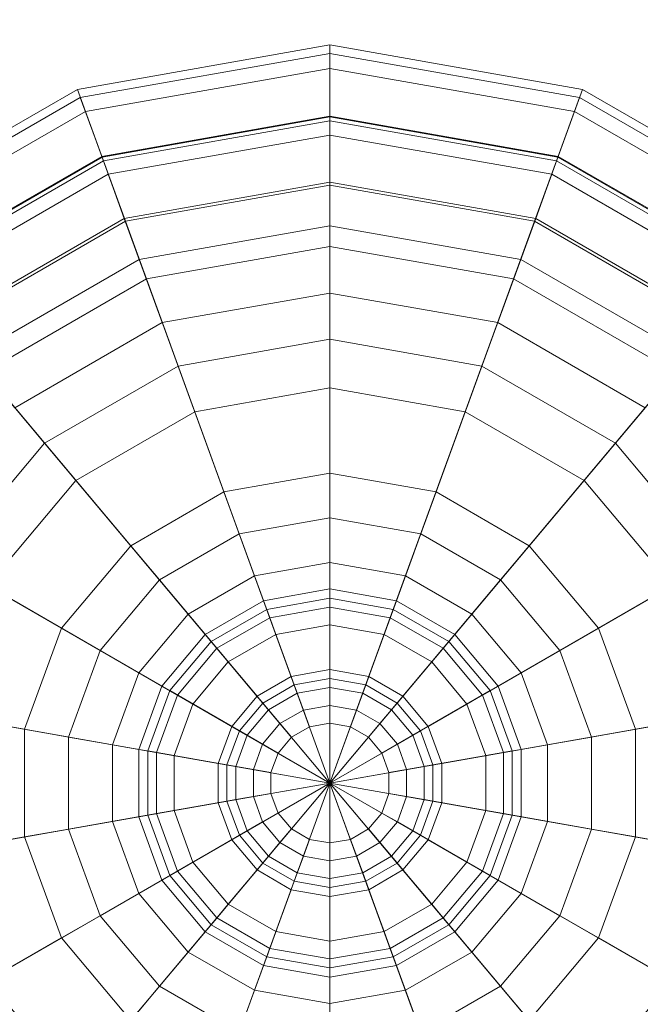
# Model space of a CAD drawing. Units: inches. Extents: x 375 to 1122, y 27 to 1069.
# Tile 92 of 155: x 729.113 to 730.25, y 860.072 to 861.878. Entities that reach past the tile are written whole.
import ezdxf

# ---------------------------------------------------------------- set-up
doc = ezdxf.new("R2010")
doc.units = ezdxf.units.IN
doc.layers.add('A-ANNO-DIMS', color=2, linetype='Continuous', lineweight=18)
doc.layers.add('Furniture', color=30, linetype='Continuous', lineweight=18)
doc.styles.get("Standard").update_dxf_attribs({"font": 'arial.ttf'})
doc.dimstyles.new('ISO-25', dxfattribs={"dimtxt": 12, "dimasz": 2.5, "dimexe": 1.5, "dimexo": 1.5, "dimtad": 1, "dimdec": 1, "dimlunit": 3, "dimtxsty": 'Standard', "dimblk": 'ARCHTICK', "dimcen": 2.5, "dimadec": 0, "dimazin": 0, "dimtfac": 1, "dimtdec": 1, "dimtmove": 0, "dimatfit": 3, "dimfxl": 1.5, "dimfxlon": 1, "dimarcsym": 0})

# ---------------------------------------------------------------- blocks, each defined once
blk = doc.blocks.new('A$C403C54AD')
for points in [[(1.940462, 1.15174, -0.060915), (1.946342, 1.118392, -0.057836), (1.946342, 1.118392, -0.057836), (1.929411, 1.147718, -0.060915)], [(1.952223, 1.15174, -0.060915), (1.946342, 1.118392, -0.057836), (1.946342, 1.118392, -0.057836), (1.940462, 1.15174, -0.060915)], [(1.963274, 1.147718, -0.060915), (1.946342, 1.118392, -0.057836), (1.946342, 1.118392, -0.057836), (1.952223, 1.15174, -0.060915)], [(1.943874, 1.13239, -0.054409), (1.941029, 1.148524, -0.057684), (1.931044, 1.144889, -0.057684), (1.939235, 1.130702, -0.054409)], [(1.948811, 1.13239, -0.054409), (1.951655, 1.148524, -0.057684), (1.941029, 1.148524, -0.057684), (1.943874, 1.13239, -0.054409)], [(1.95345, 1.130702, -0.054409), (1.961641, 1.144889, -0.057684), (1.951655, 1.148524, -0.057684), (1.948811, 1.13239, -0.054409)], [(1.929411, 1.147718, -0.060915), (1.946342, 1.118392, -0.057836), (1.946342, 1.118392, -0.057836), (1.920403, 1.140158, -0.060915)], [(1.972282, 1.140158, -0.060915), (1.946342, 1.118392, -0.057836), (1.946342, 1.118392, -0.057836), (1.963274, 1.147718, -0.060915)], [(1.939235, 1.130702, -0.054409), (1.931044, 1.144889, -0.057684), (1.922904, 1.138059, -0.057684), (1.935454, 1.127529, -0.054409)], [(1.957231, 1.127529, -0.054409), (1.969781, 1.138059, -0.057684), (1.961641, 1.144889, -0.057684), (1.95345, 1.130702, -0.054409)], [(1.932631, 1.142142, 0.042594), (1.936164, 1.136022, 0.032362), (1.930748, 1.131478, 0.032362), (1.925335, 1.13602, 0.042594)], [(1.920403, 1.140158, -0.060915), (1.946342, 1.118392, -0.057836), (1.946342, 1.118392, -0.057836), (1.914522, 1.129974, -0.060915)], [(1.922904, 1.138059, -0.057684), (1.920403, 1.140158, -0.060915), (1.914522, 1.129974, -0.060915), (1.917591, 1.128857, -0.057684)], [(1.978163, 1.129974, -0.060915), (1.946342, 1.118392, -0.057836), (1.946342, 1.118392, -0.057836), (1.972282, 1.140158, -0.060915)], [(1.922935, 1.138033, 0.102069), (1.920708, 1.139902, 0.088845), (1.914897, 1.129837, 0.088845), (1.917629, 1.128843, 0.102069)], [(1.920708, 1.139902, 0.088845), (1.921225, 1.139468, 0.060603), (1.915531, 1.129606, 0.060603), (1.914897, 1.129837, 0.088845)], [(1.937279, 1.134091, 0.03455), (1.934036, 1.139708, 0.043942), (1.927488, 1.134213, 0.043942), (1.932456, 1.130044, 0.03455)], [(1.960229, 1.130044, 0.03455), (1.965197, 1.134213, 0.043942), (1.958649, 1.139708, 0.043942), (1.955406, 1.134091, 0.03455)], [(1.921225, 1.139468, 0.060603), (1.925335, 1.13602, 0.042594), (1.920572, 1.127772, 0.042594), (1.915531, 1.129606, 0.060603)], [(1.942807, 1.13844, 0.032362), (1.944585, 1.128357, 0.024995), (1.941283, 1.127155, 0.024995), (1.936164, 1.136022, 0.032362)], [(1.949878, 1.13844, 0.032362), (1.9481, 1.128357, 0.024995), (1.944585, 1.128357, 0.024995), (1.942807, 1.13844, 0.032362)], [(1.956521, 1.136022, 0.032362), (1.951402, 1.127155, 0.024995), (1.9481, 1.128357, 0.024995), (1.949878, 1.13844, 0.032362)], [(1.935454, 1.127529, -0.054409), (1.922904, 1.138059, -0.057684), (1.917591, 1.128857, -0.057684), (1.932985, 1.123254, -0.054409)], [(1.926763, 1.134821, 0.111475), (1.922935, 1.138033, 0.102069), (1.917629, 1.128843, 0.102069), (1.922324, 1.127134, 0.111475)], [(1.923071, 1.137919, 0.088628), (1.925223, 1.136113, 0.101264), (1.920436, 1.127821, 0.101264), (1.917796, 1.128782, 0.088628)], [(1.923575, 1.137496, 0.061088), (1.923071, 1.137919, 0.088628), (1.917796, 1.128782, 0.088628), (1.918414, 1.128557, 0.061088)], [(1.927488, 1.134213, 0.043942), (1.923575, 1.137496, 0.061088), (1.918414, 1.128557, 0.061088), (1.923214, 1.12681, 0.043942)], [(1.925223, 1.136113, 0.101264), (1.929121, 1.132843, 0.111475), (1.925217, 1.126081, 0.111475), (1.920436, 1.127821, 0.101264)], [(1.936164, 1.136022, 0.032362), (1.941283, 1.127155, 0.024995), (1.938591, 1.124896, 0.024995), (1.930748, 1.131478, 0.032362)], [(1.944796, 1.127161, 0.027913), (1.943195, 1.136244, 0.03455), (1.937279, 1.134091, 0.03455), (1.94189, 1.126103, 0.027913)], [(1.947889, 1.127161, 0.027913), (1.94949, 1.136244, 0.03455), (1.943195, 1.136244, 0.03455), (1.944796, 1.127161, 0.027913)], [(1.950795, 1.126103, 0.027913), (1.955406, 1.134091, 0.03455), (1.94949, 1.136244, 0.03455), (1.947889, 1.127161, 0.027913)], [(1.961937, 1.131478, 0.032362), (1.954094, 1.124896, 0.024995), (1.951402, 1.127155, 0.024995), (1.956521, 1.136022, 0.032362)], [(1.925335, 1.13602, 0.042594), (1.930748, 1.131478, 0.032362), (1.927213, 1.125355, 0.032362), (1.920572, 1.127772, 0.042594)], [(1.929121, 1.132843, 0.111475), (1.926763, 1.134821, 0.111475), (1.922324, 1.127134, 0.111475), (1.925217, 1.126081, 0.111475)], [(1.932456, 1.130044, 0.03455), (1.927488, 1.134213, 0.043942), (1.923214, 1.12681, 0.043942), (1.929308, 1.124592, 0.03455)], [(1.94189, 1.126103, 0.027913), (1.937279, 1.134091, 0.03455), (1.932456, 1.130044, 0.03455), (1.939522, 1.124116, 0.027913)], [(1.953163, 1.124116, 0.027913), (1.960229, 1.130044, 0.03455), (1.955406, 1.134091, 0.03455), (1.950795, 1.126103, 0.027913)], [(1.94423, 1.130374, -0.051544), (1.943874, 1.13239, -0.054409), (1.939235, 1.130702, -0.054409), (1.940259, 1.128929, -0.051544)], [(1.948455, 1.130374, -0.051544), (1.948811, 1.13239, -0.054409), (1.943874, 1.13239, -0.054409), (1.94423, 1.130374, -0.051544)], [(1.952426, 1.128929, -0.051544), (1.95345, 1.130702, -0.054409), (1.948811, 1.13239, -0.054409), (1.948455, 1.130374, -0.051544)], [(1.930748, 1.131478, 0.032362), (1.938591, 1.124896, 0.024995), (1.936834, 1.121853, 0.024995), (1.927213, 1.125355, 0.032362)], [(1.965472, 1.125355, 0.032362), (1.955851, 1.121853, 0.024995), (1.954094, 1.124896, 0.024995), (1.961937, 1.131478, 0.032362)], [(1.940259, 1.128929, -0.051544), (1.939235, 1.130702, -0.054409), (1.935454, 1.127529, -0.054409), (1.937022, 1.126213, -0.051544)], [(1.955663, 1.126213, -0.051544), (1.957231, 1.127529, -0.054409), (1.95345, 1.130702, -0.054409), (1.952426, 1.128929, -0.051544)], [(1.944941, 1.12634, -0.049498), (1.94423, 1.130374, -0.051544), (1.940259, 1.128929, -0.051544), (1.942307, 1.125382, -0.049498)], [(1.947744, 1.12634, -0.049498), (1.948455, 1.130374, -0.051544), (1.94423, 1.130374, -0.051544), (1.944941, 1.12634, -0.049498)], [(1.950378, 1.125382, -0.049498), (1.952426, 1.128929, -0.051544), (1.948455, 1.130374, -0.051544), (1.947744, 1.12634, -0.049498)], [(1.914522, 1.129974, -0.060915), (1.946342, 1.118392, -0.057836), (1.946342, 1.118392, -0.057836), (1.91248, 1.118392, -0.060915)], [(1.917591, 1.128857, -0.057684), (1.914522, 1.129974, -0.060915), (1.91248, 1.118392, -0.060915), (1.915746, 1.118392, -0.057684)], [(1.917629, 1.128843, 0.102069), (1.914897, 1.129837, 0.088845), (1.912879, 1.118392, 0.088845), (1.915786, 1.118392, 0.102069)], [(1.914897, 1.129837, 0.088845), (1.915531, 1.129606, 0.060603), (1.913554, 1.118392, 0.060603), (1.912879, 1.118392, 0.088845)], [(1.939522, 1.124116, 0.027913), (1.932456, 1.130044, 0.03455), (1.929308, 1.124592, 0.03455), (1.937975, 1.121437, 0.027913)], [(1.980205, 1.118392, -0.060915), (1.946342, 1.118392, -0.057836), (1.946342, 1.118392, -0.057836), (1.978163, 1.129974, -0.060915)], [(1.95471, 1.121437, 0.027913), (1.963376, 1.124592, 0.03455), (1.960229, 1.130044, 0.03455), (1.953163, 1.124116, 0.027913)], [(1.915531, 1.129606, 0.060603), (1.920572, 1.127772, 0.042594), (1.918919, 1.118392, 0.042594), (1.913554, 1.118392, 0.060603)], [(1.932985, 1.123254, -0.054409), (1.917591, 1.128857, -0.057684), (1.915746, 1.118392, -0.057684), (1.932128, 1.118392, -0.054409)], [(1.922324, 1.127134, 0.111475), (1.917629, 1.128843, 0.102069), (1.915786, 1.118392, 0.102069), (1.920783, 1.118392, 0.111475)], [(1.942307, 1.125382, -0.049498), (1.940259, 1.128929, -0.051544), (1.937022, 1.126213, -0.051544), (1.94016, 1.12358, -0.049498)], [(1.952525, 1.12358, -0.049498), (1.955663, 1.126213, -0.051544), (1.952426, 1.128929, -0.051544), (1.950378, 1.125382, -0.049498)], [(1.917796, 1.128782, 0.088628), (1.920436, 1.127821, 0.101264), (1.918773, 1.118392, 0.101264), (1.915964, 1.118392, 0.088628)], [(1.918414, 1.128557, 0.061088), (1.917796, 1.128782, 0.088628), (1.915964, 1.118392, 0.088628), (1.916622, 1.118392, 0.061088)], [(1.923214, 1.12681, 0.043942), (1.918414, 1.128557, 0.061088), (1.916622, 1.118392, 0.061088), (1.921729, 1.118392, 0.043942)], [(1.944585, 1.128357, 0.024995), (1.945439, 1.123517, 0.024176), (1.94374, 1.122899, 0.024176), (1.941283, 1.127155, 0.024995)], [(1.9481, 1.128357, 0.024995), (1.947246, 1.123517, 0.024176), (1.945439, 1.123517, 0.024176), (1.944585, 1.128357, 0.024995)], [(1.951402, 1.127155, 0.024995), (1.948945, 1.122899, 0.024176), (1.947246, 1.123517, 0.024176), (1.9481, 1.128357, 0.024995)], [(1.920436, 1.127821, 0.101264), (1.925217, 1.126081, 0.111475), (1.923861, 1.118392, 0.111475), (1.918773, 1.118392, 0.101264)], [(1.920572, 1.127772, 0.042594), (1.927213, 1.125355, 0.032362), (1.925985, 1.118392, 0.032362), (1.918919, 1.118392, 0.042594)], [(1.937022, 1.126213, -0.051544), (1.935454, 1.127529, -0.054409), (1.932985, 1.123254, -0.054409), (1.93491, 1.122553, -0.051544)], [(1.957775, 1.122553, -0.051544), (1.9597, 1.123254, -0.054409), (1.957231, 1.127529, -0.054409), (1.955663, 1.126213, -0.051544)], [(1.925217, 1.126081, 0.111475), (1.922324, 1.127134, 0.111475), (1.920783, 1.118392, 0.111475), (1.923861, 1.118392, 0.111475)], [(1.941283, 1.127155, 0.024995), (1.94374, 1.122899, 0.024176), (1.942356, 1.121737, 0.024176), (1.938591, 1.124896, 0.024995)], [(1.946342, 1.118392, 0.02643), (1.944796, 1.127161, 0.027913), (1.94189, 1.126103, 0.027913), (1.946342, 1.118392, 0.02643)], [(1.946342, 1.118392, 0.02643), (1.947889, 1.127161, 0.027913), (1.944796, 1.127161, 0.027913), (1.946342, 1.118392, 0.02643)], [(1.946342, 1.118392, 0.02643), (1.950795, 1.126103, 0.027913), (1.947889, 1.127161, 0.027913), (1.946342, 1.118392, 0.02643)], [(1.954094, 1.124896, 0.024995), (1.950329, 1.121737, 0.024176), (1.948945, 1.122899, 0.024176), (1.951402, 1.127155, 0.024995)], [(1.929308, 1.124592, 0.03455), (1.923214, 1.12681, 0.043942), (1.921729, 1.118392, 0.043942), (1.928215, 1.118392, 0.03455)], [(1.94487, 1.126744, 0.021311), (1.945581, 1.122711, 0.019264), (1.94415, 1.12219, 0.019264), (1.942102, 1.125736, 0.021311)], [(1.945083, 1.125534, 0.023357), (1.94487, 1.126744, 0.021311), (1.942102, 1.125736, 0.021311), (1.942717, 1.124672, 0.023357)], [(1.947815, 1.126744, 0.021311), (1.947104, 1.122711, 0.019264), (1.945581, 1.122711, 0.019264), (1.94487, 1.126744, 0.021311)], [(1.947602, 1.125534, 0.023357), (1.947815, 1.126744, 0.021311), (1.94487, 1.126744, 0.021311), (1.945083, 1.125534, 0.023357)], [(1.950583, 1.125736, 0.021311), (1.948535, 1.12219, 0.019264), (1.947104, 1.122711, 0.019264), (1.947815, 1.126744, 0.021311)], [(1.949968, 1.124672, 0.023357), (1.950583, 1.125736, 0.021311), (1.947815, 1.126744, 0.021311), (1.947602, 1.125534, 0.023357)], [(1.94016, 1.12358, -0.049498), (1.937022, 1.126213, -0.051544), (1.93491, 1.122553, -0.051544), (1.938758, 1.121153, -0.049498)], [(1.946342, 1.118392, 0.02643), (1.94189, 1.126103, 0.027913), (1.939522, 1.124116, 0.027913), (1.946342, 1.118392, 0.02643)], [(1.94551, 1.123114, -0.044177), (1.944941, 1.12634, -0.049498), (1.942307, 1.125382, -0.049498), (1.943945, 1.122544, -0.044177)], [(1.947175, 1.123114, -0.044177), (1.947744, 1.12634, -0.049498), (1.944941, 1.12634, -0.049498), (1.94551, 1.123114, -0.044177)], [(1.946342, 1.118392, 0.02643), (1.953163, 1.124116, 0.027913), (1.950795, 1.126103, 0.027913), (1.946342, 1.118392, 0.02643)], [(1.94874, 1.122544, -0.044177), (1.950378, 1.125382, -0.049498), (1.947744, 1.12634, -0.049498), (1.947175, 1.123114, -0.044177)], [(1.953927, 1.121153, -0.049498), (1.957775, 1.122553, -0.051544), (1.955663, 1.126213, -0.051544), (1.952525, 1.12358, -0.049498)], [(1.942102, 1.125736, 0.021311), (1.94415, 1.12219, 0.019264), (1.942983, 1.121211, 0.019264), (1.939846, 1.123843, 0.021311)], [(1.942717, 1.124672, 0.023357), (1.942102, 1.125736, 0.021311), (1.939846, 1.123843, 0.021311), (1.940787, 1.123054, 0.023357)], [(1.952839, 1.123843, 0.021311), (1.949702, 1.121211, 0.019264), (1.948535, 1.12219, 0.019264), (1.950583, 1.125736, 0.021311)], [(1.951898, 1.123054, 0.023357), (1.952839, 1.123843, 0.021311), (1.950583, 1.125736, 0.021311), (1.949968, 1.124672, 0.023357)], [(1.927213, 1.125355, 0.032362), (1.936834, 1.121853, 0.024995), (1.936224, 1.118392, 0.024995), (1.925985, 1.118392, 0.032362)], [(1.943945, 1.122544, -0.044177), (1.942307, 1.125382, -0.049498), (1.94016, 1.12358, -0.049498), (1.94267, 1.121474, -0.044177)], [(1.945439, 1.123517, 0.024176), (1.945083, 1.125534, 0.023357), (1.942717, 1.124672, 0.023357), (1.94374, 1.122899, 0.024176)], [(1.947246, 1.123517, 0.024176), (1.947602, 1.125534, 0.023357), (1.945083, 1.125534, 0.023357), (1.945439, 1.123517, 0.024176)], [(1.948945, 1.122899, 0.024176), (1.949968, 1.124672, 0.023357), (1.947602, 1.125534, 0.023357), (1.947246, 1.123517, 0.024176)], [(1.950015, 1.121474, -0.044177), (1.952525, 1.12358, -0.049498), (1.950378, 1.125382, -0.049498), (1.94874, 1.122544, -0.044177)], [(1.9667, 1.118392, 0.032362), (1.956461, 1.118392, 0.024995), (1.955851, 1.121853, 0.024995), (1.965472, 1.125355, 0.032362)], [(1.938591, 1.124896, 0.024995), (1.942356, 1.121737, 0.024176), (1.941452, 1.120172, 0.024176), (1.936834, 1.121853, 0.024995)], [(1.955851, 1.121853, 0.024995), (1.951233, 1.120172, 0.024176), (1.950329, 1.121737, 0.024176), (1.954094, 1.124896, 0.024995)], [(1.937975, 1.121437, 0.027913), (1.929308, 1.124592, 0.03455), (1.928215, 1.118392, 0.03455), (1.937438, 1.118392, 0.027913)], [(1.94374, 1.122899, 0.024176), (1.942717, 1.124672, 0.023357), (1.940787, 1.123054, 0.023357), (1.942356, 1.121737, 0.024176)], [(1.950329, 1.121737, 0.024176), (1.951898, 1.123054, 0.023357), (1.949968, 1.124672, 0.023357), (1.948945, 1.122899, 0.024176)], [(1.955247, 1.118392, 0.027913), (1.96447, 1.118392, 0.03455), (1.963376, 1.124592, 0.03455), (1.95471, 1.121437, 0.027913)], [(1.946342, 1.118392, 0.02643), (1.939522, 1.124116, 0.027913), (1.937975, 1.121437, 0.027913), (1.946342, 1.118392, 0.02643)], [(1.939846, 1.123843, 0.021311), (1.942983, 1.121211, 0.019264), (1.942222, 1.119892, 0.019264), (1.938373, 1.121293, 0.021311)], [(1.940787, 1.123054, 0.023357), (1.939846, 1.123843, 0.021311), (1.938373, 1.121293, 0.021311), (1.939528, 1.120872, 0.023357)], [(1.946342, 1.118392, 0.02643), (1.95471, 1.121437, 0.027913), (1.953163, 1.124116, 0.027913), (1.946342, 1.118392, 0.02643)], [(1.954312, 1.121293, 0.021311), (1.950463, 1.119892, 0.019264), (1.949702, 1.121211, 0.019264), (1.952839, 1.123843, 0.021311)], [(1.953157, 1.120872, 0.023357), (1.954312, 1.121293, 0.021311), (1.952839, 1.123843, 0.021311), (1.951898, 1.123054, 0.023357)], [(1.94267, 1.121474, -0.044177), (1.94016, 1.12358, -0.049498), (1.938758, 1.121153, -0.049498), (1.941837, 1.120032, -0.044177)], [(1.950848, 1.120032, -0.044177), (1.953927, 1.121153, -0.049498), (1.952525, 1.12358, -0.049498), (1.950015, 1.121474, -0.044177)], [(1.93491, 1.122553, -0.051544), (1.932985, 1.123254, -0.054409), (1.932128, 1.118392, -0.054409), (1.934176, 1.118392, -0.051544)], [(1.942356, 1.121737, 0.024176), (1.940787, 1.123054, 0.023357), (1.939528, 1.120872, 0.023357), (1.941452, 1.120172, 0.024176)], [(1.945723, 1.121904, -0.035582), (1.94551, 1.123114, -0.044177), (1.943945, 1.122544, -0.044177), (1.94456, 1.12148, -0.035582)], [(1.946962, 1.121904, -0.035582), (1.947175, 1.123114, -0.044177), (1.94551, 1.123114, -0.044177), (1.945723, 1.121904, -0.035582)], [(1.948125, 1.12148, -0.035582), (1.94874, 1.122544, -0.044177), (1.947175, 1.123114, -0.044177), (1.946962, 1.121904, -0.035582)], [(1.951233, 1.120172, 0.024176), (1.953157, 1.120872, 0.023357), (1.951898, 1.123054, 0.023357), (1.950329, 1.121737, 0.024176)], [(1.938758, 1.121153, -0.049498), (1.93491, 1.122553, -0.051544), (1.934176, 1.118392, -0.051544), (1.938271, 1.118392, -0.049498)], [(1.94456, 1.12148, -0.035582), (1.943945, 1.122544, -0.044177), (1.94267, 1.121474, -0.044177), (1.943611, 1.120684, -0.035582)], [(1.945581, 1.122711, 0.019264), (1.945865, 1.121097, 0.012716), (1.944969, 1.120771, 0.012716), (1.94415, 1.12219, 0.019264)], [(1.947104, 1.122711, 0.019264), (1.946819, 1.121097, 0.012716), (1.945865, 1.121097, 0.012716), (1.945581, 1.122711, 0.019264)], [(1.948535, 1.12219, 0.019264), (1.947716, 1.120771, 0.012716), (1.946819, 1.121097, 0.012716), (1.947104, 1.122711, 0.019264)], [(1.949074, 1.120684, -0.035582), (1.950015, 1.121474, -0.044177), (1.94874, 1.122544, -0.044177), (1.948125, 1.12148, -0.035582)], [(1.954413, 1.118392, -0.049498), (1.958509, 1.118392, -0.051544), (1.957775, 1.122553, -0.051544), (1.953927, 1.121153, -0.049498)], [(1.94415, 1.12219, 0.019264), (1.944969, 1.120771, 0.012716), (1.944238, 1.120158, 0.012716), (1.942983, 1.121211, 0.019264)], [(1.949702, 1.121211, 0.019264), (1.948447, 1.120158, 0.012716), (1.947716, 1.120771, 0.012716), (1.948535, 1.12219, 0.019264)], [(1.936834, 1.121853, 0.024995), (1.941452, 1.120172, 0.024176), (1.941138, 1.118392, 0.024176), (1.936224, 1.118392, 0.024995)], [(1.945865, 1.121097, 0.012716), (1.945723, 1.121904, -0.035582), (1.94456, 1.12148, -0.035582), (1.944969, 1.120771, 0.012716)], [(1.946819, 1.121097, 0.012716), (1.946962, 1.121904, -0.035582), (1.945723, 1.121904, -0.035582), (1.945865, 1.121097, 0.012716)], [(1.947716, 1.120771, 0.012716), (1.948125, 1.12148, -0.035582), (1.946962, 1.121904, -0.035582), (1.946819, 1.121097, 0.012716)], [(1.956461, 1.118392, 0.024995), (1.951547, 1.118392, 0.024176), (1.951233, 1.120172, 0.024176), (1.955851, 1.121853, 0.024995)], [(1.946342, 1.118392, 0.02643), (1.937975, 1.121437, 0.027913), (1.937438, 1.118392, 0.027913), (1.946342, 1.118392, 0.02643)], [(1.938373, 1.121293, 0.021311), (1.942222, 1.119892, 0.019264), (1.941957, 1.118392, 0.019264), (1.937862, 1.118392, 0.021311)], [(1.939528, 1.120872, 0.023357), (1.938373, 1.121293, 0.021311), (1.937862, 1.118392, 0.021311), (1.939091, 1.118392, 0.023357)], [(1.941837, 1.120032, -0.044177), (1.938758, 1.121153, -0.049498), (1.938271, 1.118392, -0.049498), (1.941548, 1.118392, -0.044177)], [(1.943611, 1.120684, -0.035582), (1.94267, 1.121474, -0.044177), (1.941837, 1.120032, -0.044177), (1.942992, 1.119612, -0.035582)], [(1.942983, 1.121211, 0.019264), (1.944238, 1.120158, 0.012716), (1.943761, 1.119332, 0.012716), (1.942222, 1.119892, 0.019264)], [(1.944969, 1.120771, 0.012716), (1.94456, 1.12148, -0.035582), (1.943611, 1.120684, -0.035582), (1.944238, 1.120158, 0.012716)], [(1.946342, 1.118392, 0.02643), (1.955247, 1.118392, 0.027913), (1.95471, 1.121437, 0.027913), (1.946342, 1.118392, 0.02643)], [(1.948447, 1.120158, 0.012716), (1.949074, 1.120684, -0.035582), (1.948125, 1.12148, -0.035582), (1.947716, 1.120771, 0.012716)], [(1.950463, 1.119892, 0.019264), (1.948924, 1.119332, 0.012716), (1.948447, 1.120158, 0.012716), (1.949702, 1.121211, 0.019264)], [(1.949693, 1.119612, -0.035582), (1.950848, 1.120032, -0.044177), (1.950015, 1.121474, -0.044177), (1.949074, 1.120684, -0.035582)], [(1.954823, 1.118392, 0.021311), (1.950727, 1.118392, 0.019264), (1.950463, 1.119892, 0.019264), (1.954312, 1.121293, 0.021311)], [(1.951137, 1.118392, -0.044177), (1.954413, 1.118392, -0.049498), (1.953927, 1.121153, -0.049498), (1.950848, 1.120032, -0.044177)], [(1.953594, 1.118392, 0.023357), (1.954823, 1.118392, 0.021311), (1.954312, 1.121293, 0.021311), (1.953157, 1.120872, 0.023357)], [(1.941452, 1.120172, 0.024176), (1.939528, 1.120872, 0.023357), (1.939091, 1.118392, 0.023357), (1.941138, 1.118392, 0.024176)], [(1.944238, 1.120158, 0.012716), (1.943611, 1.120684, -0.035582), (1.942992, 1.119612, -0.035582), (1.943761, 1.119332, 0.012716)], [(1.948924, 1.119332, 0.012716), (1.949693, 1.119612, -0.035582), (1.949074, 1.120684, -0.035582), (1.948447, 1.120158, 0.012716)], [(1.951547, 1.118392, 0.024176), (1.953594, 1.118392, 0.023357), (1.953157, 1.120872, 0.023357), (1.951233, 1.120172, 0.024176)], [(1.942992, 1.119612, -0.035582), (1.941837, 1.120032, -0.044177), (1.941548, 1.118392, -0.044177), (1.942777, 1.118392, -0.035582)], [(1.942222, 1.119892, 0.019264), (1.943761, 1.119332, 0.012716), (1.943596, 1.118392, 0.012716), (1.941957, 1.118392, 0.019264)], [(1.950727, 1.118392, 0.019264), (1.949089, 1.118392, 0.012716), (1.948924, 1.119332, 0.012716), (1.950463, 1.119892, 0.019264)], [(1.949908, 1.118392, -0.035582), (1.951137, 1.118392, -0.044177), (1.950848, 1.120032, -0.044177), (1.949693, 1.119612, -0.035582)], [(1.943761, 1.119332, 0.012716), (1.942992, 1.119612, -0.035582), (1.942777, 1.118392, -0.035582), (1.943596, 1.118392, 0.012716)], [(1.949089, 1.118392, 0.012716), (1.949908, 1.118392, -0.035582), (1.949693, 1.119612, -0.035582), (1.948924, 1.119332, 0.012716)], [(1.91248, 1.118392, -0.060915), (1.946342, 1.118392, -0.057836), (1.946342, 1.118392, -0.057836), (1.914522, 1.106811, -0.060915)], [(1.915746, 1.118392, -0.057684), (1.91248, 1.118392, -0.060915), (1.914522, 1.106811, -0.060915), (1.917591, 1.107928, -0.057684)], [(1.915786, 1.118392, 0.102069), (1.912879, 1.118392, 0.088845), (1.914897, 1.106947, 0.088845), (1.917629, 1.107941, 0.102069)], [(1.912879, 1.118392, 0.088845), (1.913554, 1.118392, 0.060603), (1.915531, 1.107178, 0.060603), (1.914897, 1.106947, 0.088845)], [(1.913554, 1.118392, 0.060603), (1.918919, 1.118392, 0.042594), (1.920572, 1.109013, 0.042594), (1.915531, 1.107178, 0.060603)], [(1.914522, 1.106811, -0.060915), (1.946342, 1.118392, -0.057836), (1.946342, 1.118392, -0.057836), (1.920403, 1.096626, -0.060915)], [(1.932128, 1.118392, -0.054409), (1.915746, 1.118392, -0.057684), (1.917591, 1.107928, -0.057684), (1.932985, 1.113531, -0.054409)], [(1.920783, 1.118392, 0.111475), (1.915786, 1.118392, 0.102069), (1.917629, 1.107941, 0.102069), (1.922324, 1.10965, 0.111475)], [(1.915964, 1.118392, 0.088628), (1.918773, 1.118392, 0.101264), (1.920436, 1.108963, 0.101264), (1.917796, 1.108002, 0.088628)], [(1.916622, 1.118392, 0.061088), (1.915964, 1.118392, 0.088628), (1.917796, 1.108002, 0.088628), (1.918414, 1.108227, 0.061088)], [(1.921729, 1.118392, 0.043942), (1.916622, 1.118392, 0.061088), (1.918414, 1.108227, 0.061088), (1.923214, 1.109974, 0.043942)], [(1.918773, 1.118392, 0.101264), (1.923861, 1.118392, 0.111475), (1.925217, 1.110703, 0.111475), (1.920436, 1.108963, 0.101264)], [(1.918919, 1.118392, 0.042594), (1.925985, 1.118392, 0.032362), (1.927213, 1.111429, 0.032362), (1.920572, 1.109013, 0.042594)], [(1.920403, 1.096626, -0.060915), (1.946342, 1.118392, -0.057836), (1.946342, 1.118392, -0.057836), (1.929411, 1.089067, -0.060915)], [(1.923861, 1.118392, 0.111475), (1.920783, 1.118392, 0.111475), (1.922324, 1.10965, 0.111475), (1.925217, 1.110703, 0.111475)], [(1.928215, 1.118392, 0.03455), (1.921729, 1.118392, 0.043942), (1.923214, 1.109974, 0.043942), (1.929308, 1.112192, 0.03455)], [(1.925985, 1.118392, 0.032362), (1.936224, 1.118392, 0.024995), (1.936834, 1.114931, 0.024995), (1.927213, 1.111429, 0.032362)], [(1.937438, 1.118392, 0.027913), (1.928215, 1.118392, 0.03455), (1.929308, 1.112192, 0.03455), (1.937975, 1.115347, 0.027913)], [(1.929411, 1.089067, -0.060915), (1.946342, 1.118392, -0.057836), (1.946342, 1.118392, -0.057836), (1.940462, 1.085044, -0.060915)], [(1.934176, 1.118392, -0.051544), (1.932128, 1.118392, -0.054409), (1.932985, 1.113531, -0.054409), (1.93491, 1.114231, -0.051544)], [(1.938271, 1.118392, -0.049498), (1.934176, 1.118392, -0.051544), (1.93491, 1.114231, -0.051544), (1.938758, 1.115632, -0.049498)], [(1.936224, 1.118392, 0.024995), (1.941138, 1.118392, 0.024176), (1.941452, 1.116612, 0.024176), (1.936834, 1.114931, 0.024995)], [(1.946342, 1.118392, 0.02643), (1.937438, 1.118392, 0.027913), (1.937975, 1.115347, 0.027913), (1.946342, 1.118392, 0.02643)], [(1.937862, 1.118392, 0.021311), (1.941957, 1.118392, 0.019264), (1.942222, 1.116892, 0.019264), (1.938373, 1.115492, 0.021311)], [(1.939091, 1.118392, 0.023357), (1.937862, 1.118392, 0.021311), (1.938373, 1.115492, 0.021311), (1.939528, 1.115912, 0.023357)], [(1.946342, 1.118392, 0.02643), (1.937975, 1.115347, 0.027913), (1.939522, 1.112669, 0.027913), (1.946342, 1.118392, 0.02643)], [(1.941548, 1.118392, -0.044177), (1.938271, 1.118392, -0.049498), (1.938758, 1.115632, -0.049498), (1.941837, 1.116752, -0.044177)], [(1.941138, 1.118392, 0.024176), (1.939091, 1.118392, 0.023357), (1.939528, 1.115912, 0.023357), (1.941452, 1.116612, 0.024176)], [(1.946342, 1.118392, 0.02643), (1.939522, 1.112669, 0.027913), (1.94189, 1.110681, 0.027913), (1.946342, 1.118392, 0.02643)], [(1.940462, 1.085044, -0.060915), (1.946342, 1.118392, -0.057836), (1.946342, 1.118392, -0.057836), (1.952223, 1.085044, -0.060915)], [(1.942777, 1.118392, -0.035582), (1.941548, 1.118392, -0.044177), (1.941837, 1.116752, -0.044177), (1.942992, 1.117172, -0.035582)], [(1.946342, 1.118392, 0.02643), (1.94189, 1.110681, 0.027913), (1.944796, 1.109623, 0.027913), (1.946342, 1.118392, 0.02643)], [(1.941957, 1.118392, 0.019264), (1.943596, 1.118392, 0.012716), (1.943761, 1.117453, 0.012716), (1.942222, 1.116892, 0.019264)], [(1.943596, 1.118392, 0.012716), (1.942777, 1.118392, -0.035582), (1.942992, 1.117172, -0.035582), (1.943761, 1.117453, 0.012716)], [(1.946342, 1.118392, 0.02643), (1.944796, 1.109623, 0.027913), (1.947889, 1.109623, 0.027913), (1.946342, 1.118392, 0.02643)], [(1.946342, 1.118392, 0.02643), (1.95471, 1.115347, 0.027913), (1.955247, 1.118392, 0.027913), (1.946342, 1.118392, 0.02643)], [(1.946342, 1.118392, 0.02643), (1.953163, 1.112669, 0.027913), (1.95471, 1.115347, 0.027913), (1.946342, 1.118392, 0.02643)], [(1.946342, 1.118392, 0.02643), (1.950795, 1.110681, 0.027913), (1.953163, 1.112669, 0.027913), (1.946342, 1.118392, 0.02643)], [(1.946342, 1.118392, 0.02643), (1.947889, 1.109623, 0.027913), (1.950795, 1.110681, 0.027913), (1.946342, 1.118392, 0.02643)], [(1.972282, 1.096626, -0.060915), (1.946342, 1.118392, -0.057836), (1.946342, 1.118392, -0.057836), (1.978163, 1.106811, -0.060915)], [(1.963274, 1.089067, -0.060915), (1.946342, 1.118392, -0.057836), (1.946342, 1.118392, -0.057836), (1.972282, 1.096626, -0.060915)], [(1.952223, 1.085044, -0.060915), (1.946342, 1.118392, -0.057836), (1.946342, 1.118392, -0.057836), (1.963274, 1.089067, -0.060915)], [(1.978163, 1.106811, -0.060915), (1.946342, 1.118392, -0.057836), (1.946342, 1.118392, -0.057836), (1.980205, 1.118392, -0.060915)], [(1.950463, 1.116892, 0.019264), (1.948924, 1.117453, 0.012716), (1.949089, 1.118392, 0.012716), (1.950727, 1.118392, 0.019264)], [(1.948924, 1.117453, 0.012716), (1.949693, 1.117172, -0.035582), (1.949908, 1.118392, -0.035582), (1.949089, 1.118392, 0.012716)], [(1.949693, 1.117172, -0.035582), (1.950848, 1.116752, -0.044177), (1.951137, 1.118392, -0.044177), (1.949908, 1.118392, -0.035582)], [(1.954312, 1.115492, 0.021311), (1.950463, 1.116892, 0.019264), (1.950727, 1.118392, 0.019264), (1.954823, 1.118392, 0.021311)], [(1.950848, 1.116752, -0.044177), (1.953927, 1.115632, -0.049498), (1.954413, 1.118392, -0.049498), (1.951137, 1.118392, -0.044177)], [(1.951233, 1.116612, 0.024176), (1.953157, 1.115912, 0.023357), (1.953594, 1.118392, 0.023357), (1.951547, 1.118392, 0.024176)], [(1.955851, 1.114931, 0.024995), (1.951233, 1.116612, 0.024176), (1.951547, 1.118392, 0.024176), (1.956461, 1.118392, 0.024995)], [(1.953157, 1.115912, 0.023357), (1.954312, 1.115492, 0.021311), (1.954823, 1.118392, 0.021311), (1.953594, 1.118392, 0.023357)], [(1.953927, 1.115632, -0.049498), (1.957775, 1.114231, -0.051544), (1.958509, 1.118392, -0.051544), (1.954413, 1.118392, -0.049498)], [(1.95471, 1.115347, 0.027913), (1.963376, 1.112192, 0.03455), (1.96447, 1.118392, 0.03455), (1.955247, 1.118392, 0.027913)], [(1.965472, 1.111429, 0.032362), (1.955851, 1.114931, 0.024995), (1.956461, 1.118392, 0.024995), (1.9667, 1.118392, 0.032362)], [(1.942992, 1.117172, -0.035582), (1.941837, 1.116752, -0.044177), (1.94267, 1.11531, -0.044177), (1.943611, 1.1161, -0.035582)], [(1.942222, 1.116892, 0.019264), (1.943761, 1.117453, 0.012716), (1.944238, 1.116626, 0.012716), (1.942983, 1.115573, 0.019264)], [(1.943761, 1.117453, 0.012716), (1.942992, 1.117172, -0.035582), (1.943611, 1.1161, -0.035582), (1.944238, 1.116626, 0.012716)], [(1.949702, 1.115573, 0.019264), (1.948447, 1.116626, 0.012716), (1.948924, 1.117453, 0.012716), (1.950463, 1.116892, 0.019264)], [(1.948447, 1.116626, 0.012716), (1.949074, 1.1161, -0.035582), (1.949693, 1.117172, -0.035582), (1.948924, 1.117453, 0.012716)], [(1.949074, 1.1161, -0.035582), (1.950015, 1.11531, -0.044177), (1.950848, 1.116752, -0.044177), (1.949693, 1.117172, -0.035582)], [(1.936834, 1.114931, 0.024995), (1.941452, 1.116612, 0.024176), (1.942356, 1.115047, 0.024176), (1.938591, 1.111888, 0.024995)], [(1.938373, 1.115492, 0.021311), (1.942222, 1.116892, 0.019264), (1.942983, 1.115573, 0.019264), (1.939846, 1.112941, 0.021311)], [(1.941837, 1.116752, -0.044177), (1.938758, 1.115632, -0.049498), (1.94016, 1.113204, -0.049498), (1.94267, 1.11531, -0.044177)], [(1.941452, 1.116612, 0.024176), (1.939528, 1.115912, 0.023357), (1.940787, 1.113731, 0.023357), (1.942356, 1.115047, 0.024176)], [(1.942983, 1.115573, 0.019264), (1.944238, 1.116626, 0.012716), (1.944969, 1.116013, 0.012716), (1.94415, 1.114595, 0.019264)], [(1.944238, 1.116626, 0.012716), (1.943611, 1.1161, -0.035582), (1.94456, 1.115304, -0.035582), (1.944969, 1.116013, 0.012716)], [(1.948535, 1.114595, 0.019264), (1.947716, 1.116013, 0.012716), (1.948447, 1.116626, 0.012716), (1.949702, 1.115573, 0.019264)], [(1.947716, 1.116013, 0.012716), (1.948125, 1.115304, -0.035582), (1.949074, 1.1161, -0.035582), (1.948447, 1.116626, 0.012716)], [(1.952839, 1.112941, 0.021311), (1.949702, 1.115573, 0.019264), (1.950463, 1.116892, 0.019264), (1.954312, 1.115492, 0.021311)], [(1.950015, 1.11531, -0.044177), (1.952525, 1.113204, -0.049498), (1.953927, 1.115632, -0.049498), (1.950848, 1.116752, -0.044177)], [(1.950329, 1.115047, 0.024176), (1.951898, 1.113731, 0.023357), (1.953157, 1.115912, 0.023357), (1.951233, 1.116612, 0.024176)], [(1.954094, 1.111888, 0.024995), (1.950329, 1.115047, 0.024176), (1.951233, 1.116612, 0.024176), (1.955851, 1.114931, 0.024995)], [(1.939528, 1.115912, 0.023357), (1.938373, 1.115492, 0.021311), (1.939846, 1.112941, 0.021311), (1.940787, 1.113731, 0.023357)], [(1.943611, 1.1161, -0.035582), (1.94267, 1.11531, -0.044177), (1.943945, 1.11424, -0.044177), (1.94456, 1.115304, -0.035582)], [(1.94415, 1.114595, 0.019264), (1.944969, 1.116013, 0.012716), (1.945865, 1.115687, 0.012716), (1.945581, 1.114074, 0.019264)], [(1.944969, 1.116013, 0.012716), (1.94456, 1.115304, -0.035582), (1.945723, 1.11488, -0.035582), (1.945865, 1.115687, 0.012716)], [(1.947104, 1.114074, 0.019264), (1.946819, 1.115687, 0.012716), (1.947716, 1.116013, 0.012716), (1.948535, 1.114595, 0.019264)], [(1.946819, 1.115687, 0.012716), (1.946962, 1.11488, -0.035582), (1.948125, 1.115304, -0.035582), (1.947716, 1.116013, 0.012716)], [(1.948125, 1.115304, -0.035582), (1.94874, 1.11424, -0.044177), (1.950015, 1.11531, -0.044177), (1.949074, 1.1161, -0.035582)], [(1.951898, 1.113731, 0.023357), (1.952839, 1.112941, 0.021311), (1.954312, 1.115492, 0.021311), (1.953157, 1.115912, 0.023357)], [(1.937975, 1.115347, 0.027913), (1.929308, 1.112192, 0.03455), (1.932456, 1.10674, 0.03455), (1.939522, 1.112669, 0.027913)], [(1.938758, 1.115632, -0.049498), (1.93491, 1.114231, -0.051544), (1.937022, 1.110572, -0.051544), (1.94016, 1.113204, -0.049498)], [(1.939846, 1.112941, 0.021311), (1.942983, 1.115573, 0.019264), (1.94415, 1.114595, 0.019264), (1.942102, 1.111048, 0.021311)], [(1.94267, 1.11531, -0.044177), (1.94016, 1.113204, -0.049498), (1.942307, 1.111402, -0.049498), (1.943945, 1.11424, -0.044177)], [(1.94456, 1.115304, -0.035582), (1.943945, 1.11424, -0.044177), (1.94551, 1.11367, -0.044177), (1.945723, 1.11488, -0.035582)], [(1.945581, 1.114074, 0.019264), (1.945865, 1.115687, 0.012716), (1.946819, 1.115687, 0.012716), (1.947104, 1.114074, 0.019264)], [(1.945865, 1.115687, 0.012716), (1.945723, 1.11488, -0.035582), (1.946962, 1.11488, -0.035582), (1.946819, 1.115687, 0.012716)], [(1.946962, 1.11488, -0.035582), (1.947175, 1.11367, -0.044177), (1.94874, 1.11424, -0.044177), (1.948125, 1.115304, -0.035582)], [(1.950583, 1.111048, 0.021311), (1.948535, 1.114595, 0.019264), (1.949702, 1.115573, 0.019264), (1.952839, 1.112941, 0.021311)], [(1.94874, 1.11424, -0.044177), (1.950378, 1.111402, -0.049498), (1.952525, 1.113204, -0.049498), (1.950015, 1.11531, -0.044177)], [(1.952525, 1.113204, -0.049498), (1.955663, 1.110572, -0.051544), (1.957775, 1.114231, -0.051544), (1.953927, 1.115632, -0.049498)], [(1.953163, 1.112669, 0.027913), (1.960229, 1.10674, 0.03455), (1.963376, 1.112192, 0.03455), (1.95471, 1.115347, 0.027913)], [(1.927213, 1.111429, 0.032362), (1.936834, 1.114931, 0.024995), (1.938591, 1.111888, 0.024995), (1.930748, 1.105307, 0.032362)], [(1.938591, 1.111888, 0.024995), (1.942356, 1.115047, 0.024176), (1.94374, 1.113885, 0.024176), (1.941283, 1.109629, 0.024995)], [(1.942356, 1.115047, 0.024176), (1.940787, 1.113731, 0.023357), (1.942717, 1.112112, 0.023357), (1.94374, 1.113885, 0.024176)], [(1.945723, 1.11488, -0.035582), (1.94551, 1.11367, -0.044177), (1.947175, 1.11367, -0.044177), (1.946962, 1.11488, -0.035582)], [(1.948945, 1.113885, 0.024176), (1.949968, 1.112112, 0.023357), (1.951898, 1.113731, 0.023357), (1.950329, 1.115047, 0.024176)], [(1.951402, 1.109629, 0.024995), (1.948945, 1.113885, 0.024176), (1.950329, 1.115047, 0.024176), (1.954094, 1.111888, 0.024995)], [(1.961937, 1.105307, 0.032362), (1.954094, 1.111888, 0.024995), (1.955851, 1.114931, 0.024995), (1.965472, 1.111429, 0.032362)], [(1.942102, 1.111048, 0.021311), (1.94415, 1.114595, 0.019264), (1.945581, 1.114074, 0.019264), (1.94487, 1.11004, 0.021311)], [(1.947815, 1.11004, 0.021311), (1.947104, 1.114074, 0.019264), (1.948535, 1.114595, 0.019264), (1.950583, 1.111048, 0.021311)], [(1.93491, 1.114231, -0.051544), (1.932985, 1.113531, -0.054409), (1.935454, 1.109255, -0.054409), (1.937022, 1.110572, -0.051544)], [(1.943945, 1.11424, -0.044177), (1.942307, 1.111402, -0.049498), (1.944941, 1.110444, -0.049498), (1.94551, 1.11367, -0.044177)], [(1.94487, 1.11004, 0.021311), (1.945581, 1.114074, 0.019264), (1.947104, 1.114074, 0.019264), (1.947815, 1.11004, 0.021311)], [(1.947175, 1.11367, -0.044177), (1.947744, 1.110444, -0.049498), (1.950378, 1.111402, -0.049498), (1.94874, 1.11424, -0.044177)], [(1.955663, 1.110572, -0.051544), (1.957231, 1.109255, -0.054409), (1.9597, 1.113531, -0.054409), (1.957775, 1.114231, -0.051544)], [(1.932985, 1.113531, -0.054409), (1.917591, 1.107928, -0.057684), (1.922904, 1.098725, -0.057684), (1.935454, 1.109255, -0.054409)], [(1.940787, 1.113731, 0.023357), (1.939846, 1.112941, 0.021311), (1.942102, 1.111048, 0.021311), (1.942717, 1.112112, 0.023357)], [(1.941283, 1.109629, 0.024995), (1.94374, 1.113885, 0.024176), (1.945439, 1.113267, 0.024176), (1.944585, 1.108427, 0.024995)], [(1.94374, 1.113885, 0.024176), (1.942717, 1.112112, 0.023357), (1.945083, 1.11125, 0.023357), (1.945439, 1.113267, 0.024176)], [(1.94551, 1.11367, -0.044177), (1.944941, 1.110444, -0.049498), (1.947744, 1.110444, -0.049498), (1.947175, 1.11367, -0.044177)], [(1.947246, 1.113267, 0.024176), (1.947602, 1.11125, 0.023357), (1.949968, 1.112112, 0.023357), (1.948945, 1.113885, 0.024176)], [(1.9481, 1.108427, 0.024995), (1.947246, 1.113267, 0.024176), (1.948945, 1.113885, 0.024176), (1.951402, 1.109629, 0.024995)], [(1.949968, 1.112112, 0.023357), (1.950583, 1.111048, 0.021311), (1.952839, 1.112941, 0.021311), (1.951898, 1.113731, 0.023357)], [(1.94016, 1.113204, -0.049498), (1.937022, 1.110572, -0.051544), (1.940259, 1.107856, -0.051544), (1.942307, 1.111402, -0.049498)], [(1.944585, 1.108427, 0.024995), (1.945439, 1.113267, 0.024176), (1.947246, 1.113267, 0.024176), (1.9481, 1.108427, 0.024995)], [(1.945439, 1.113267, 0.024176), (1.945083, 1.11125, 0.023357), (1.947602, 1.11125, 0.023357), (1.947246, 1.113267, 0.024176)], [(1.950378, 1.111402, -0.049498), (1.952426, 1.107856, -0.051544), (1.955663, 1.110572, -0.051544), (1.952525, 1.113204, -0.049498)], [(1.939522, 1.112669, 0.027913), (1.932456, 1.10674, 0.03455), (1.937279, 1.102693, 0.03455), (1.94189, 1.110681, 0.027913)], [(1.950795, 1.110681, 0.027913), (1.955406, 1.102693, 0.03455), (1.960229, 1.10674, 0.03455), (1.953163, 1.112669, 0.027913)], [(1.929308, 1.112192, 0.03455), (1.923214, 1.109974, 0.043942), (1.927488, 1.102571, 0.043942), (1.932456, 1.10674, 0.03455)], [(1.942717, 1.112112, 0.023357), (1.942102, 1.111048, 0.021311), (1.94487, 1.11004, 0.021311), (1.945083, 1.11125, 0.023357)], [(1.947602, 1.11125, 0.023357), (1.947815, 1.11004, 0.021311), (1.950583, 1.111048, 0.021311), (1.949968, 1.112112, 0.023357)], [(1.930748, 1.105307, 0.032362), (1.938591, 1.111888, 0.024995), (1.941283, 1.109629, 0.024995), (1.936164, 1.100762, 0.032362)], [(1.956521, 1.100762, 0.032362), (1.951402, 1.109629, 0.024995), (1.954094, 1.111888, 0.024995), (1.961937, 1.105307, 0.032362)], [(1.920572, 1.109013, 0.042594), (1.927213, 1.111429, 0.032362), (1.930748, 1.105307, 0.032362), (1.925335, 1.100764, 0.042594)], [(1.942307, 1.111402, -0.049498), (1.940259, 1.107856, -0.051544), (1.94423, 1.10641, -0.051544), (1.944941, 1.110444, -0.049498)], [(1.945083, 1.11125, 0.023357), (1.94487, 1.11004, 0.021311), (1.947815, 1.11004, 0.021311), (1.947602, 1.11125, 0.023357)], [(1.947744, 1.110444, -0.049498), (1.948455, 1.10641, -0.051544), (1.952426, 1.107856, -0.051544), (1.950378, 1.111402, -0.049498)], [(1.920436, 1.108963, 0.101264), (1.925217, 1.110703, 0.111475), (1.929121, 1.103941, 0.111475), (1.925223, 1.100671, 0.101264)], [(1.925217, 1.110703, 0.111475), (1.922324, 1.10965, 0.111475), (1.926763, 1.101963, 0.111475), (1.929121, 1.103941, 0.111475)], [(1.937022, 1.110572, -0.051544), (1.935454, 1.109255, -0.054409), (1.939235, 1.106082, -0.054409), (1.940259, 1.107856, -0.051544)], [(1.94189, 1.110681, 0.027913), (1.937279, 1.102693, 0.03455), (1.943195, 1.10054, 0.03455), (1.944796, 1.109623, 0.027913)], [(1.944941, 1.110444, -0.049498), (1.94423, 1.10641, -0.051544), (1.948455, 1.10641, -0.051544), (1.947744, 1.110444, -0.049498)], [(1.947889, 1.109623, 0.027913), (1.94949, 1.10054, 0.03455), (1.955406, 1.102693, 0.03455), (1.950795, 1.110681, 0.027913)], [(1.952426, 1.107856, -0.051544), (1.95345, 1.106082, -0.054409), (1.957231, 1.109255, -0.054409), (1.955663, 1.110572, -0.051544)], [(1.923214, 1.109974, 0.043942), (1.918414, 1.108227, 0.061088), (1.923575, 1.099288, 0.061088), (1.927488, 1.102571, 0.043942)], [(1.922324, 1.10965, 0.111475), (1.917629, 1.107941, 0.102069), (1.922935, 1.098751, 0.102069), (1.926763, 1.101963, 0.111475)], [(1.936164, 1.100762, 0.032362), (1.941283, 1.109629, 0.024995), (1.944585, 1.108427, 0.024995), (1.942807, 1.098344, 0.032362)], [(1.944796, 1.109623, 0.027913), (1.943195, 1.10054, 0.03455), (1.94949, 1.10054, 0.03455), (1.947889, 1.109623, 0.027913)], [(1.949878, 1.098344, 0.032362), (1.9481, 1.108427, 0.024995), (1.951402, 1.109629, 0.024995), (1.956521, 1.100762, 0.032362)], [(1.915531, 1.107178, 0.060603), (1.920572, 1.109013, 0.042594), (1.925335, 1.100764, 0.042594), (1.921225, 1.097316, 0.060603)], [(1.917796, 1.108002, 0.088628), (1.920436, 1.108963, 0.101264), (1.925223, 1.100671, 0.101264), (1.923071, 1.098865, 0.088628)], [(1.935454, 1.109255, -0.054409), (1.922904, 1.098725, -0.057684), (1.931044, 1.091895, -0.057684), (1.939235, 1.106082, -0.054409)], [(1.95345, 1.106082, -0.054409), (1.961641, 1.091895, -0.057684), (1.969781, 1.098725, -0.057684), (1.957231, 1.109255, -0.054409)], [(1.918414, 1.108227, 0.061088), (1.917796, 1.108002, 0.088628), (1.923071, 1.098865, 0.088628), (1.923575, 1.099288, 0.061088)], [(1.942807, 1.098344, 0.032362), (1.944585, 1.108427, 0.024995), (1.9481, 1.108427, 0.024995), (1.949878, 1.098344, 0.032362)], [(1.917591, 1.107928, -0.057684), (1.914522, 1.106811, -0.060915), (1.920403, 1.096626, -0.060915), (1.922904, 1.098725, -0.057684)], [(1.917629, 1.107941, 0.102069), (1.914897, 1.106947, 0.088845), (1.920708, 1.096882, 0.088845), (1.922935, 1.098751, 0.102069)], [(1.940259, 1.107856, -0.051544), (1.939235, 1.106082, -0.054409), (1.943874, 1.104394, -0.054409), (1.94423, 1.10641, -0.051544)], [(1.948455, 1.10641, -0.051544), (1.948811, 1.104394, -0.054409), (1.95345, 1.106082, -0.054409), (1.952426, 1.107856, -0.051544)], [(1.914897, 1.106947, 0.088845), (1.915531, 1.107178, 0.060603), (1.921225, 1.097316, 0.060603), (1.920708, 1.096882, 0.088845)], [(1.932456, 1.10674, 0.03455), (1.927488, 1.102571, 0.043942), (1.934036, 1.097077, 0.043942), (1.937279, 1.102693, 0.03455)], [(1.955406, 1.102693, 0.03455), (1.958649, 1.097077, 0.043942), (1.965197, 1.102571, 0.043942), (1.960229, 1.10674, 0.03455)], [(1.94423, 1.10641, -0.051544), (1.943874, 1.104394, -0.054409), (1.948811, 1.104394, -0.054409), (1.948455, 1.10641, -0.051544)], [(1.939235, 1.106082, -0.054409), (1.931044, 1.091895, -0.057684), (1.941029, 1.088261, -0.057684), (1.943874, 1.104394, -0.054409)], [(1.948811, 1.104394, -0.054409), (1.951655, 1.088261, -0.057684), (1.961641, 1.091895, -0.057684), (1.95345, 1.106082, -0.054409)], [(1.925335, 1.100764, 0.042594), (1.930748, 1.105307, 0.032362), (1.936164, 1.100762, 0.032362), (1.932631, 1.094642, 0.042594)], [(1.943874, 1.104394, -0.054409), (1.941029, 1.088261, -0.057684), (1.951655, 1.088261, -0.057684), (1.948811, 1.104394, -0.054409)]]:
    blk.add_3dface(points)
blk = doc.blocks.new('_ArchTick')
at = {"color": 0, "linetype": 'ByBlock', "const_width": 0.15}
blk.add_lwpolyline([(-0.5, -0.5), (0.5, 0.5)], dxfattribs=at)
blk = doc.blocks.new('*D85')
at = {"layer": 'A-ANNO-DIMS', "color": 0, "lineweight": -2, "transparency": 16777216}
for p, q in [((401.5073, 868.5277), (398.5073, 868.5277)), ((400.0073, 814.5277), (400.0073, 868.5277)), ((401.5073, 814.5277), (398.5073, 814.5277))]:
    blk.add_line(p, q, dxfattribs=at)
at = {"layer": 'Defpoints', "color": 0, "transparency": 16777216}
for p in [(400.0073, 868.5277), (845.0073, 868.5277), (845.0073, 814.5277)]:
    blk.add_point(p, dxfattribs=at)
at = {"layer": 'A-ANNO-DIMS', "color": 0, "lineweight": -2, "transparency": 16777216, "xscale": 2.5, "yscale": 2.5, "zscale": 2.5}
for p, rotation in [((400.0073, 868.5277), 90), ((400.0073, 814.5277), 270)]:
    blk.add_blockref('_ArchTick', p, dxfattribs=dict(at, rotation=rotation))
at = {"layer": 'A-ANNO-DIMS', "color": 0, "transparency": 16777216, "insert": (393.2555, 841.5277), "char_height": 12, "attachment_point": 5, "rotation": 90}
blk.add_mtext('4\'-6"', dxfattribs=at)
blk = doc.blocks.new('*D88')
at = {"layer": 'A-ANNO-DIMS', "color": 0, "lineweight": -2, "transparency": 16777216}
for p, q in [((731.0073, 1052.5277), (731.0073, 1055.5277)), ((854.0073, 1052.5277), (854.0073, 1055.5277)), ((731.0073, 1054.0277), (854.0073, 1054.0277))]:
    blk.add_line(p, q, dxfattribs=at)
at = {"layer": 'Defpoints', "color": 0, "transparency": 16777216}
for p in [(854.0073, 1054.0277), (731.0073, 502.5277), (854.0073, 502.5277)]:
    blk.add_point(p, dxfattribs=at)
at = {"layer": 'A-ANNO-DIMS', "color": 0, "lineweight": -2, "transparency": 16777216, "xscale": 2.5, "yscale": 2.5, "zscale": 2.5, "rotation": 180}
blk.add_blockref('_ArchTick', (731.0073, 1054.0277), dxfattribs=at)
at = {"layer": 'A-ANNO-DIMS', "color": 0, "lineweight": -2, "transparency": 16777216, "xscale": 2.5, "yscale": 2.5, "zscale": 2.5}
blk.add_blockref('_ArchTick', (854.0073, 1054.0277), dxfattribs=at)
at = {"layer": 'A-ANNO-DIMS', "color": 0, "transparency": 16777216, "insert": (792.5073, 1060.7837), "char_height": 12, "attachment_point": 5}
blk.add_mtext('10\'-3"', dxfattribs=at)
blk = doc.blocks.new('*D91')
at = {"layer": 'A-ANNO-DIMS', "color": 0, "lineweight": -2, "transparency": 16777216}
for p, q in [((728.0073, 1052.5277), (728.0073, 1055.5277)), ((788.0073, 1052.5277), (788.0073, 1055.5277)), ((728.0073, 1054.0277), (788.0073, 1054.0277))]:
    blk.add_line(p, q, dxfattribs=at)
at = {"layer": 'Defpoints', "color": 0, "transparency": 16777216}
for p in [(788.0073, 1054.0277), (728.0073, 774.0277), (788.0073, 774.0277)]:
    blk.add_point(p, dxfattribs=at)
at = {"layer": 'A-ANNO-DIMS', "color": 0, "lineweight": -2, "transparency": 16777216, "xscale": 2.5, "yscale": 2.5, "zscale": 2.5, "rotation": 180}
blk.add_blockref('_ArchTick', (728.0073, 1054.0277), dxfattribs=at)
at = {"layer": 'A-ANNO-DIMS', "color": 0, "lineweight": -2, "transparency": 16777216, "xscale": 2.5, "yscale": 2.5, "zscale": 2.5}
blk.add_blockref('_ArchTick', (788.0073, 1054.0277), dxfattribs=at)
at = {"layer": 'A-ANNO-DIMS', "color": 0, "transparency": 16777216, "insert": (758.0073, 1060.7796), "char_height": 12, "attachment_point": 5}
blk.add_mtext('5\'-0"', dxfattribs=at)

msp = doc.modelspace()

# ---------------------------------------------------------------- block references
at = {"layer": 'Furniture', "xscale": 39.9918517141215, "yscale": 39.9918517141215, "zscale": 39.9918517141215, "rotation": 270}
msp.add_blockref('A$C403C54AD', (684.9549, 938.3156, 0.024), dxfattribs=at)

# ---------------------------------------------------------------- dimensions: what is measured, and where the dimension line sits
at = {"layer": 'A-ANNO-DIMS'}
for base, p1, p2, picture, middle in [((788.0073, 1054.0277), (728.0073, 774.0277), (788.0073, 774.0277), '*D91', (758.0073, 1060.7796)), ((854.0073, 1054.0277), (731.0073, 502.5277), (854.0073, 502.5277), '*D88', (792.5073, 1060.7837))]:
    dim = msp.add_linear_dim(base=base, p1=p1, p2=p2, dimstyle='ISO-25', override={"dimdec": 1, "dimlfac": 1, "dimrnd": 0, "dimzin": 1, "dimdsep": 46, "dimlunit": 4, "dimfrac": 2}, dxfattribs=at)
    dim.commit()
    dim.dimension.update_dxf_attribs({"geometry": picture, "text_midpoint": middle})
dim = msp.add_linear_dim(base=(400.0073, 868.5277), p1=(845.0073, 814.5277), p2=(845.0073, 868.5277), angle=90, dimstyle='ISO-25', override={"dimdec": 1, "dimlfac": 1, "dimrnd": 0, "dimzin": 1, "dimdsep": 46, "dimlunit": 4, "dimfrac": 2}, dxfattribs=at)
dim.commit()
dim.dimension.update_dxf_attribs({"geometry": '*D85', "text_midpoint": (393.2555, 841.5277)})

doc.saveas('drawing.dxf')
